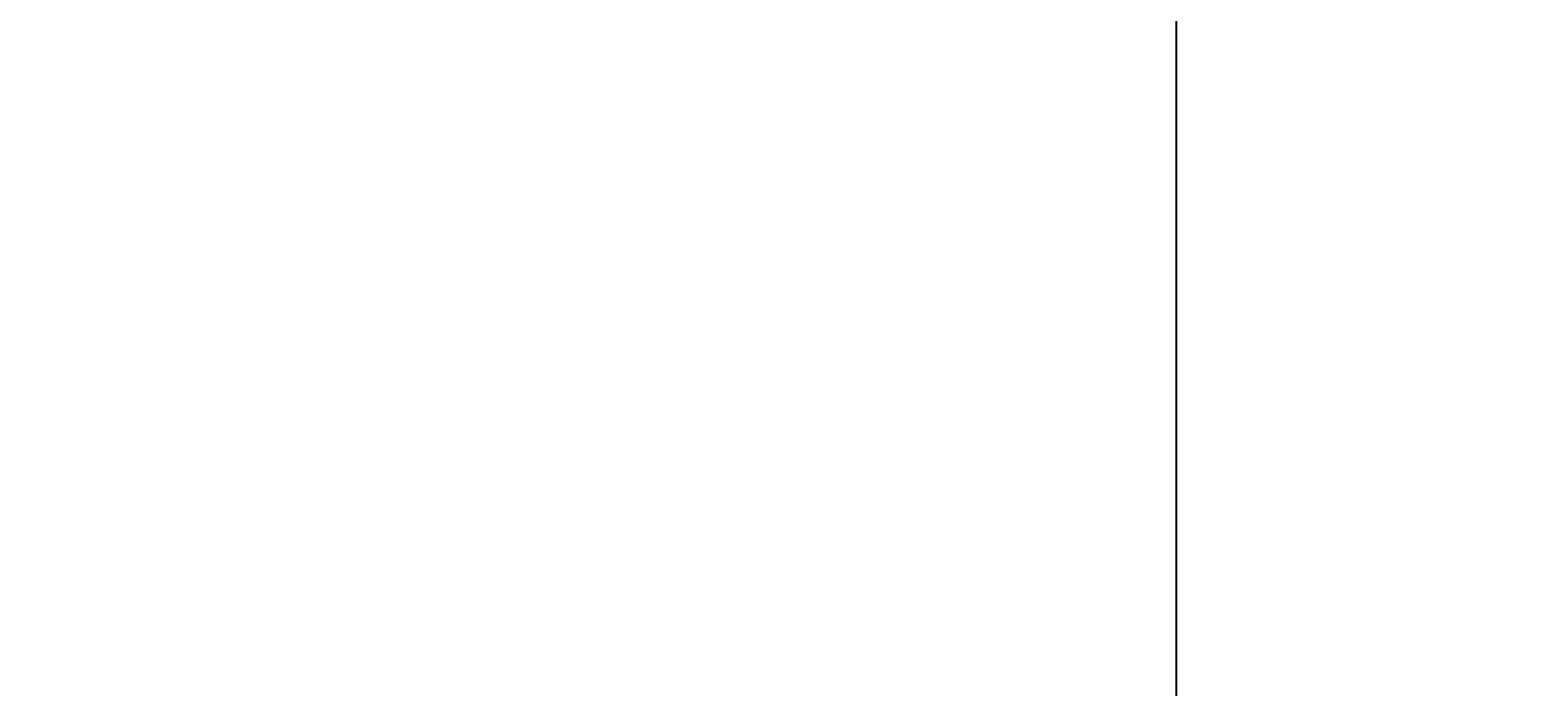
# Model space of a CAD drawing. Units: inches. Extents: x 35362 to 73946, y 43607 to 67532.
# Tile 54 of 134: x 49302 to 50119, y 46564 to 46919. Entities that reach past the tile are written whole.
import ezdxf

# ---------------------------------------------------------------- set-up
doc = ezdxf.new("R2010")
doc.units = ezdxf.units.IN
doc.header["$MEASUREMENT"] = 0
doc.layers.add('A-ANNO-DIMS', color=2, linetype='Continuous', lineweight=18)
doc.styles.get("Standard").update_dxf_attribs({"font": 'arial.ttf'})
doc.dimstyles.get("Standard").update_dxf_attribs({"dimtxt": 0.18, "dimasz": 0.18, "dimexe": 0.18, "dimexo": 0.0625, "dimgap": 0.09, "dimtad": 0, "dimtih": 1, "dimtoh": 1, "dimdec": 4, "dimzin": 0, "dimdsep": 46, "dimtxsty": 'Standard', "dimcen": 0.09, "dimadec": 0, "dimazin": 0, "dimtfac": 1, "dimtdec": 4, "dimtofl": 0, "dimtmove": 0, "dimatfit": 3, "dimfxl": 1, "dimtolj": 1, "dimtzin": 0, "dimarcsym": 0})

# ---------------------------------------------------------------- blocks, each defined once
blk = doc.blocks.new('*D5')
at = {"layer": 'A-ANNO-DIMS', "color": 0, "lineweight": -2, "transparency": 16777216}
for p, q in [((37121.95, 46919.32), (37121.95, 43606.68)), ((69871.5, 45449.83), (69871.5, 43606.68)), ((37122.13, 43606.86), (53496.29, 43606.86)), ((69871.32, 43606.86), (53497.15, 43606.86))]:
    blk.add_line(p, q, dxfattribs=at)
at = {"layer": 'A-ANNO-DIMS', "color": 0, "transparency": 16777216}
for points in [[(37122.13, 43606.89), (37122.13, 43606.83), (37121.95, 43606.86)], [(69871.32, 43606.89), (69871.32, 43606.83), (69871.5, 43606.86)]]:
    blk.add_solid(points, dxfattribs=at)
at = {"layer": 'Defpoints', "color": 0, "transparency": 16777216}
for p in [(37121.95, 46919.38), (69871.5, 45449.89), (69871.5, 43606.86)]:
    blk.add_point(p, dxfattribs=at)
at = {"layer": 'A-ANNO-DIMS', "color": 0, "transparency": 16777216, "insert": (53496.72, 43606.86), "char_height": 0.18, "attachment_point": 5}
blk.add_mtext('\\A1;32750', dxfattribs=at)
blk = doc.blocks.new('*D11')
at = {"layer": 'A-ANNO-DIMS', "color": 0, "lineweight": -2, "transparency": 16777216}
for p, q in [((47978.66, 56028.77), (47978.66, 43606.68)), ((53109.76, 56028.77), (53109.76, 43606.68)), ((47978.84, 43606.86), (50543.87, 43606.86)), ((53109.58, 43606.86), (50544.55, 43606.86))]:
    blk.add_line(p, q, dxfattribs=at)
at = {"layer": 'A-ANNO-DIMS', "color": 0, "transparency": 16777216}
for points in [[(47978.84, 43606.89), (47978.84, 43606.83), (47978.66, 43606.86)], [(53109.58, 43606.89), (53109.58, 43606.83), (53109.76, 43606.86)]]:
    blk.add_solid(points, dxfattribs=at)
at = {"layer": 'Defpoints', "color": 0, "transparency": 16777216}
for p in [(47978.66, 56028.84), (53109.76, 56028.84), (53109.76, 43606.86)]:
    blk.add_point(p, dxfattribs=at)
at = {"layer": 'A-ANNO-DIMS', "color": 0, "transparency": 16777216, "insert": (50544.21, 43606.86), "char_height": 0.18, "attachment_point": 5}
blk.add_mtext('\\A1;5131', dxfattribs=at)
blk = doc.blocks.new('*D13')
at = {"layer": 'A-ANNO-DIMS', "color": 0, "lineweight": -2, "transparency": 16777216}
for p, q in [((48373.49, 51694.02), (48373.49, 43606.68)), ((51029.04, 51694.02), (51029.04, 43606.68)), ((48373.67, 43606.86), (49700.8, 43606.86)), ((51028.86, 43606.86), (49701.73, 43606.86))]:
    blk.add_line(p, q, dxfattribs=at)
at = {"layer": 'A-ANNO-DIMS', "color": 0, "transparency": 16777216}
for points in [[(48373.67, 43606.89), (48373.67, 43606.83), (48373.49, 43606.86)], [(51028.86, 43606.89), (51028.86, 43606.83), (51029.04, 43606.86)]]:
    blk.add_solid(points, dxfattribs=at)
at = {"layer": 'Defpoints', "color": 0, "transparency": 16777216}
for p in [(48373.49, 51694.09), (51029.04, 51694.09), (51029.04, 43606.86)]:
    blk.add_point(p, dxfattribs=at)
at = {"layer": 'A-ANNO-DIMS', "color": 0, "transparency": 16777216, "insert": (49701.27, 43606.86), "char_height": 0.18, "attachment_point": 5}
blk.add_mtext('\\A1;2655.6', dxfattribs=at)
blk = doc.blocks.new('*D17')
at = {"layer": 'A-ANNO-DIMS', "color": 0, "lineweight": -2, "transparency": 16777216}
for p, q in [((49923.31, 61293.22), (49923.31, 43606.68)), ((51913.93, 61293.22), (51913.93, 43606.68)), ((49923.49, 43606.86), (50918.16, 43606.86)), ((51913.75, 43606.86), (50919.07, 43606.86))]:
    blk.add_line(p, q, dxfattribs=at)
at = {"layer": 'A-ANNO-DIMS', "color": 0, "transparency": 16777216}
for points in [[(49923.49, 43606.89), (49923.49, 43606.83), (49923.31, 43606.86)], [(51913.75, 43606.89), (51913.75, 43606.83), (51913.93, 43606.86)]]:
    blk.add_solid(points, dxfattribs=at)
at = {"layer": 'Defpoints', "color": 0, "transparency": 16777216}
for p in [(49923.31, 61293.29), (51913.93, 61293.29), (51913.93, 43606.86)]:
    blk.add_point(p, dxfattribs=at)
at = {"layer": 'A-ANNO-DIMS', "color": 0, "transparency": 16777216, "insert": (50918.62, 43606.86), "char_height": 0.18, "attachment_point": 5}
blk.add_mtext('\\A1;1990.6', dxfattribs=at)
blk = doc.blocks.new('*D67')
at = {"layer": 'A-ANNO-DIMS', "color": 0, "lineweight": -2, "transparency": 16777216}
for p, q in [((56873.54, 53351.53), (35361.77, 53351.53)), ((35361.95, 53351.35), (35361.95, 49400.89)), ((35361.95, 45450.07), (35361.95, 49400.53)), ((53793.58, 45449.89), (35361.77, 45449.89))]:
    blk.add_line(p, q, dxfattribs=at)
at = {"layer": 'A-ANNO-DIMS', "color": 0, "transparency": 16777216}
for points in [[(35361.92, 53351.35), (35361.98, 53351.35), (35361.95, 53351.53)], [(35361.92, 45450.07), (35361.98, 45450.07), (35361.95, 45449.89)]]:
    blk.add_solid(points, dxfattribs=at)
at = {"layer": 'Defpoints', "color": 0, "transparency": 16777216}
for p in [(35361.95, 53351.53), (56873.6, 53351.53), (53793.64, 45449.89)]:
    blk.add_point(p, dxfattribs=at)
at = {"layer": 'A-ANNO-DIMS', "color": 0, "transparency": 16777216, "insert": (35361.95, 49400.71), "char_height": 0.18, "attachment_point": 5}
blk.add_mtext('\\A1;7901.6', dxfattribs=at)
blk = doc.blocks.new('*D90')
at = {"layer": 'A-ANNO-DIMS', "color": 0, "lineweight": -2, "transparency": 16777216}
for p, q in [((53707.72, 47291.29), (35361.77, 47291.29)), ((35361.95, 47291.11), (35361.95, 46710.26)), ((35361.95, 46129.06), (35361.95, 46709.9)), ((53793.58, 46128.88), (35361.77, 46128.88))]:
    blk.add_line(p, q, dxfattribs=at)
at = {"layer": 'A-ANNO-DIMS', "color": 0, "transparency": 16777216}
for points in [[(35361.92, 47291.11), (35361.98, 47291.11), (35361.95, 47291.29)], [(35361.92, 46129.06), (35361.98, 46129.06), (35361.95, 46128.88)]]:
    blk.add_solid(points, dxfattribs=at)
at = {"layer": 'Defpoints', "color": 0, "transparency": 16777216}
for p in [(53707.78, 47291.29), (35361.95, 46128.88), (53793.64, 46128.88)]:
    blk.add_point(p, dxfattribs=at)
at = {"layer": 'A-ANNO-DIMS', "color": 0, "transparency": 16777216, "insert": (35361.95, 46710.08), "char_height": 0.18, "attachment_point": 5}
blk.add_mtext('\\A1;1162.4', dxfattribs=at)

msp = doc.modelspace()

# ---------------------------------------------------------------- dimensions: what is measured, and where the dimension line sits
at = {"layer": 'A-ANNO-DIMS'}
for base, p1, p2, override, picture, middle in [((51913.931, 43606.859), (49923.307, 61293.286), (51913.931, 61293.286), {"dimdec": 1, "dimlfac": 1, "dimrnd": 0, "dimzin": 0, "dimdsep": 46, "dimlunit": 2}, '*D17', (50918.619, 43606.859)), ((53109.76, 43606.859), (47978.665, 56028.836), (53109.76, 56028.836), {"dimdec": 0, "dimlfac": 1, "dimrnd": 0, "dimzin": 0, "dimdsep": 46, "dimlunit": 2}, '*D11', (50544.212, 43606.859)), ((51029.043, 43606.859), (48373.492, 51694.087), (51029.043, 51694.087), {"dimdec": 1, "dimlfac": 1, "dimrnd": 0, "dimzin": 0, "dimdsep": 46, "dimlunit": 2}, '*D13', (49701.267, 43606.859)), ((69871.496, 43606.859), (37121.949, 46919.381), (69871.496, 45449.894), {"dimdec": 0, "dimlfac": 1, "dimrnd": 0, "dimzin": 0, "dimdsep": 46, "dimlunit": 2}, '*D5', (53496.723, 43606.859))]:
    dim = msp.add_linear_dim(base=base, p1=p1, p2=p2, dimstyle='Standard', override=override, dxfattribs=at)
    dim.commit()
    dim.dimension.update_dxf_attribs({"geometry": picture, "text_midpoint": middle})
for base, p1, p2, picture, middle in [((35361.949, 53351.529), (53793.638, 45449.894), (56873.602, 53351.529), '*D67', (35361.949, 49400.712)), ((35361.949, 46128.878), (53707.781, 47291.285), (53793.638, 46128.878), '*D90', (35361.949, 46710.081))]:
    dim = msp.add_linear_dim(base=base, p1=p1, p2=p2, angle=90, dimstyle='Standard', override={"dimdec": 1, "dimlfac": 1, "dimrnd": 0, "dimzin": 0, "dimdsep": 46, "dimlunit": 2}, dxfattribs=at)
    dim.commit()
    dim.dimension.update_dxf_attribs({"geometry": picture, "text_midpoint": middle})

doc.saveas('drawing.dxf')
